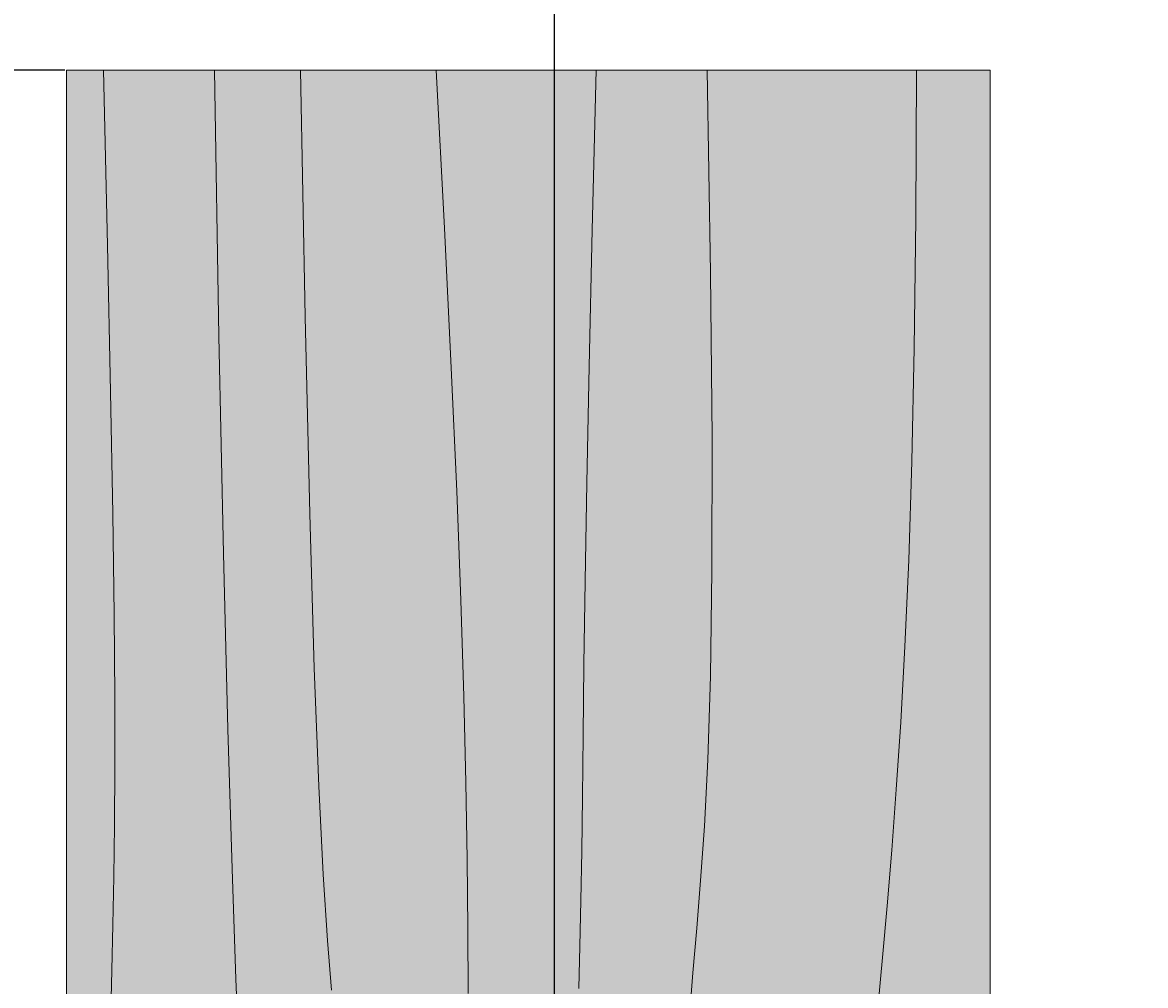
# Model space of a CAD drawing. Units: inches. Extents: x 2549 to 3108, y 1683 to 2362.
# Tile 26 of 30: x 2949 to 2985, y 2049 to 2080. Entities that reach past the tile are written whole.
import ezdxf

# ---------------------------------------------------------------- set-up
doc = ezdxf.new("R2010")
doc.units = ezdxf.units.IN
for name, color, linetype, lineweight in [('A-ANNO-DIMS', 2, 'Continuous', 18), ('A-FURN', 8, 'Continuous', 18), ('A-FURN-PATT', 9, 'Continuous', 13)]:
    doc.layers.add(name, color=color, linetype=linetype, lineweight=lineweight)
doc.layers.add('C-PKNG-VEHI-PATT', color=251, linetype='Continuous', lineweight=13, true_color=0x636466)
doc.layers.add('C-PVMT-PATT', color=9, linetype='Continuous', lineweight=13, true_color=0xc7c8ca)
doc.styles.get("Standard").update_dxf_attribs({"font": 'arial.ttf'})
doc.dimstyles.get("Standard").update_dxf_attribs({"dimtxt": 0.18, "dimasz": 0.18, "dimexe": 0.18, "dimexo": 0.0625, "dimgap": 0.09, "dimtad": 0, "dimtih": 1, "dimtoh": 1, "dimdec": 4, "dimzin": 0, "dimdsep": 46, "dimtxsty": 'Standard', "dimcen": 0.09, "dimadec": 0, "dimazin": 0, "dimtfac": 1, "dimtdec": 4, "dimtofl": 0, "dimtmove": 0, "dimatfit": 3, "dimfxl": 1, "dimtolj": 1, "dimtzin": 0, "dimarcsym": 0})

# ---------------------------------------------------------------- blocks, each defined once
blk = doc.blocks.new('Table - Rectangular Woodgrain 60 x 30 in.')
for p, q in [((0, 0), (0, -30)), ((60, 0), (0, 0)), ((0, -30), (60, -30))]:
    blk.add_line(p, q)
for points in [[(0, -2.4), (4.8155, -2.418), (9.0302, -2.4688), (12.709, -2.5477), (15.9167, -2.65), (18.7181, -2.7711), (21.1781, -2.9063), (23.3616, -3.0508), (25.3333, -3.2), (27.1477, -3.3495), (28.8172, -3.4958), (30.3437, -3.636)], [(0, -9.2), (6.5759, -9.0858), (11.9385, -9.0365), (16.2527, -9.0418), (19.6833, -9.0917), (22.3952, -9.1759), (24.5531, -9.2844), (26.322, -9.4069), (27.8666, -9.5333), (29.3241, -9.6553), (30.7203, -9.7719)], [(0, -12.8), (5.1847, -12.9322), (9.6213, -13.0323), (13.3963, -13.1059), (16.5958, -13.1583), (19.3063, -13.1952), (21.614, -13.2219), (23.6054, -13.2439), (25.3666, -13.2667), (26.9728, -13.2947), (28.4531, -13.3281), (29.8256, -13.3663)], [(0, -18), (5.124, -17.7273), (9.6609, -17.5057), (13.6705, -17.3303), (17.2125, -17.1958), (20.3467, -17.0973), (23.1328, -17.0297), (25.6307, -16.9878), (27.9, -16.9667), (29.9928, -16.9617)], [(0, -22.4), (8.0098, -22.2501), (14.4094, -22.1011), (19.4168, -21.9535), (23.25, -21.8083), (26.1269, -21.6663), (28.2656, -21.5281), (29.884, -21.3947)], [(0, -25.2), (8.6355, -25.0504), (15.7026, -24.9031), (21.4049, -24.7606), (25.9458, -24.625), (29.529, -24.4988), (32.3578, -24.3844)], [(0, -28.8), (5.6867, -28.6681), (10.45, -28.5698), (14.407, -28.5012), (17.675, -28.4584), (20.3711, -28.4374), (22.6125, -28.4344), (24.5164, -28.4455), (26.2, -28.4667), (27.762, -28.4947), (29.2276, -28.5281), (30.6033, -28.5663)]]:
    blk.add_lwpolyline(points)
blk = doc.blocks.new('*D22')
at = {"layer": 'A-ANNO-DIMS', "color": 0, "lineweight": -2, "transparency": 16777216}
for p, q in [((2950.031, 2078.615), (2940.913, 2078.615)), ((2941.093, 2078.435), (2941.093, 2048.798)), ((2941.093, 2018.795), (2941.093, 2048.431)), ((2950.031, 2018.615), (2940.913, 2018.615))]:
    blk.add_line(p, q, dxfattribs=at)
at = {"layer": 'A-ANNO-DIMS', "color": 0, "transparency": 16777216}
for points in [[(2941.063, 2078.435), (2941.123, 2078.435), (2941.093, 2078.615)], [(2941.063, 2018.795), (2941.123, 2018.795), (2941.093, 2018.615)]]:
    blk.add_solid(points, dxfattribs=at)
at = {"layer": 'Defpoints', "color": 0, "transparency": 16777216}
for p in [(2950.093, 2078.615), (2941.093, 2018.615), (2950.093, 2018.615)]:
    blk.add_point(p, dxfattribs=at)
at = {"layer": 'A-ANNO-DIMS', "color": 0, "transparency": 16777216, "insert": (2941.093, 2048.615), "char_height": 0.18, "attachment_point": 5}
blk.add_mtext('\\A1;COFFEE TABLE 60', dxfattribs=at)
blk = doc.blocks.new('*D46')
at = {"layer": 'A-ANNO-DIMS', "color": 0, "lineweight": -2, "transparency": 16777216}
for p, q in [((2812.643, 2140.461), (2812.643, 1683.444)), ((3034.643, 2134.461), (3034.643, 1683.444)), ((2812.823, 1683.624), (2923.353, 1683.624)), ((3034.463, 1683.624), (2923.932, 1683.624))]:
    blk.add_line(p, q, dxfattribs=at)
at = {"layer": 'A-ANNO-DIMS', "color": 0, "transparency": 16777216}
for points in [[(2812.823, 1683.654), (2812.823, 1683.594), (2812.643, 1683.624)], [(3034.463, 1683.654), (3034.463, 1683.594), (3034.643, 1683.624)]]:
    blk.add_solid(points, dxfattribs=at)
at = {"layer": 'Defpoints', "color": 0, "transparency": 16777216}
for p in [(2812.643, 2140.524), (3034.643, 2134.524), (3034.643, 1683.624)]:
    blk.add_point(p, dxfattribs=at)
at = {"layer": 'A-ANNO-DIMS', "color": 0, "transparency": 16777216, "insert": (2923.643, 1683.624), "char_height": 0.18, "attachment_point": 5}
blk.add_mtext('\\A1;222', dxfattribs=at)
blk = doc.blocks.new('*D57')
at = {"layer": 'A-ANNO-DIMS', "color": 0, "lineweight": -2, "transparency": 16777216}
for p, q in [((2965.935, 1936.586), (2965.935, 2362.323)), ((3034.643, 1936.586), (3034.643, 2362.323)), ((2966.115, 2362.143), (2999.912, 2362.143)), ((3034.463, 2362.143), (3000.666, 2362.143))]:
    blk.add_line(p, q, dxfattribs=at)
at = {"layer": 'A-ANNO-DIMS', "color": 0, "transparency": 16777216}
for points in [[(2966.115, 2362.173), (2966.115, 2362.113), (2965.935, 2362.143)], [(3034.463, 2362.173), (3034.463, 2362.113), (3034.643, 2362.143)]]:
    blk.add_solid(points, dxfattribs=at)
at = {"layer": 'Defpoints', "color": 0, "transparency": 16777216}
for p in [(3034.643, 2362.143), (2965.935, 1936.524), (3034.643, 1936.524)]:
    blk.add_point(p, dxfattribs=at)
at = {"layer": 'A-ANNO-DIMS', "color": 0, "transparency": 16777216, "insert": (3000.289, 2362.143), "char_height": 0.18, "attachment_point": 5}
blk.add_mtext('\\A1;68.71', dxfattribs=at)
blk = doc.blocks.new('*D63')
at = {"layer": 'A-ANNO-DIMS', "color": 0, "lineweight": -2, "transparency": 16777216}
for p, q in [((2963.328, 2197.213), (2963.508, 2197.213)), ((2963.508, 2197.213), (2963.508, 2124.675)), ((2963.419, 2003.299), (2963.599, 2003.299)), ((2963.509, 2003.209), (2963.509, 2003.389))]:
    blk.add_line(p, q, dxfattribs=at)
at = {"layer": 'A-ANNO-DIMS', "color": 0, "transparency": 16777216}
blk.add_solid([(2963.538, 2124.675), (2963.478, 2124.675), (2963.508, 2124.495)], dxfattribs=at)
at = {"layer": 'Defpoints', "color": 0, "transparency": 16777216}
for p in [(2963.508, 2124.495), (2963.509, 2003.299)]:
    blk.add_point(p, dxfattribs=at)
at = {"layer": 'A-ANNO-DIMS', "color": 0, "transparency": 16777216, "insert": (2962.654, 2197.213), "char_height": 0.18, "attachment_point": 5}
blk.add_mtext('\\A1;2X R121.2', dxfattribs=at)
blk = doc.blocks.new('*D64')
at = {"layer": 'A-ANNO-DIMS', "color": 0, "lineweight": -2, "transparency": 16777216}
for p, q in [((2919.097, 2052.001), (2919.097, 2052.181)), ((2919.007, 2052.091), (2919.187, 2052.091)), ((3101.897, 2052.091), (3033.527, 2052.091))]:
    blk.add_line(p, q, dxfattribs=at)
at = {"layer": 'A-ANNO-DIMS', "color": 0, "transparency": 16777216}
blk.add_solid([(3033.527, 2052.121), (3033.527, 2052.061), (3033.347, 2052.091)], dxfattribs=at)
at = {"layer": 'Defpoints', "color": 0, "transparency": 16777216}
for p in [(2919.097, 2052.091), (3033.347, 2052.091)]:
    blk.add_point(p, dxfattribs=at)
at = {"layer": 'A-ANNO-DIMS', "color": 0, "transparency": 16777216, "insert": (3102.642, 2052.091), "char_height": 0.18, "attachment_point": 5}
blk.add_mtext('\\A1;2X R114.25', dxfattribs=at)

msp = doc.modelspace()

# ---------------------------------------------------------------- hatches: boundary and pattern name
at = {"layer": 'A-FURN-PATT', "transparency": 33554684}
h = msp.add_hatch(color=256, dxfattribs=at)
h.dxf.hatch_style = 1
h.paths.add_polyline_path([(2951.6587, 2056.0021), (2951.6557, 2058.2435), (2951.6347, 2060.9396), (2951.5919, 2064.2076), (2951.5233, 2068.1646), (2951.425, 2072.9279), (2951.2931, 2078.6146), (2950.0931, 2078.6146), (2950.0931, 2018.6146), (2952.4931, 2018.6146), (2952.0883, 2021.7874), (2951.7676, 2024.5157), (2951.521, 2026.8517), (2951.3389, 2028.848), (2951.2115, 2030.5567), (2951.129, 2032.0303), (2951.0817, 2033.321), (2951.0598, 2034.4813), (2951.0547, 2035.5574), (2951.0634, 2036.5714), (2951.0838, 2037.5393), (2951.1139, 2038.4771), (2951.1519, 2039.4009), (2951.1957, 2040.3266), (2951.2434, 2041.2703), (2951.2931, 2042.248), (2951.343, 2043.2741), (2951.392, 2044.3568), (2951.4396, 2045.5028), (2951.4847, 2046.7188), (2951.5268, 2048.0113), (2951.565, 2049.387), (2951.5984, 2050.8526), (2951.6264, 2052.4146), (2951.6476, 2054.0982)])
h.paths.add_polyline_path([(2955.3325, 2057.2097), (2955.19, 2062.912), (2955.0427, 2069.9791), (2954.8931, 2078.6146), (2951.2931, 2078.6146), (2951.425, 2072.9279), (2951.5233, 2068.1646), (2951.5919, 2064.2076), (2951.6347, 2060.9396), (2951.6557, 2058.2435), (2951.6587, 2056.0021), (2951.6476, 2054.0982), (2951.6264, 2052.4146), (2951.5984, 2050.8526), (2951.565, 2049.387), (2951.5268, 2048.0113), (2951.4847, 2046.7188), (2951.4396, 2045.5028), (2951.392, 2044.3568), (2951.343, 2043.2741), (2951.2931, 2042.248), (2951.2434, 2041.2703), (2951.1957, 2040.3266), (2951.1519, 2039.4009), (2951.1139, 2038.4771), (2951.0838, 2037.5393), (2951.0634, 2036.5714), (2951.0547, 2035.5574), (2951.0598, 2034.4813), (2951.0817, 2033.321), (2951.129, 2032.0303), (2951.2115, 2030.5567), (2951.3389, 2028.848), (2951.521, 2026.8517), (2951.7676, 2024.5157), (2952.0883, 2021.7874), (2952.4931, 2018.6146), (2955.2931, 2018.6146), (2955.302, 2019.3711), (2955.3269, 2020.1382), (2955.3652, 2020.9125), (2955.4139, 2021.6907), (2955.4705, 2022.4692), (2955.5321, 2023.2447), (2955.5961, 2024.0137), (2955.6597, 2024.7729), (2955.7206, 2025.5211), (2955.778, 2026.2663), (2955.8314, 2027.0187), (2955.8806, 2027.7886), (2955.9251, 2028.5862), (2955.9644, 2029.4218), (2955.9984, 2030.3056), (2956.0264, 2031.2479), (2956.048, 2032.2589), (2956.0618, 2033.3479), (2956.0663, 2034.5245), (2956.0598, 2035.7979), (2956.0408, 2037.1776), (2956.0077, 2038.6729), (2955.959, 2040.2933), (2955.8931, 2042.0479), (2955.8091, 2043.9787), (2955.7087, 2046.2568), (2955.5943, 2049.0856), (2955.4681, 2052.6688)])
h.paths.add_polyline_path([(2958.1396, 2059.1978), (2957.992, 2064.2052), (2957.843, 2070.6048), (2957.6931, 2078.6146), (2954.8931, 2078.6146), (2955.0427, 2069.9791), (2955.19, 2062.912), (2955.3325, 2057.2097), (2955.4681, 2052.6688), (2955.5943, 2049.0856), (2955.7087, 2046.2568), (2955.8091, 2043.9787), (2955.8931, 2042.0479), (2955.959, 2040.2933), (2956.0077, 2038.6729), (2956.0408, 2037.1776), (2956.0598, 2035.7979), (2956.0663, 2034.5245), (2956.0618, 2033.3479), (2956.048, 2032.2589), (2956.0264, 2031.2479), (2955.9984, 2030.3056), (2955.9644, 2029.4218), (2955.9251, 2028.5862), (2955.8806, 2027.7886), (2955.8314, 2027.0187), (2955.778, 2026.2663), (2955.7206, 2025.5211), (2955.6597, 2024.7729), (2955.5961, 2024.0137), (2955.5321, 2023.2447), (2955.4705, 2022.4692), (2955.4139, 2021.6907), (2955.3652, 2020.9125), (2955.3269, 2020.1382), (2955.302, 2019.3711), (2955.2931, 2018.6146), (2958.4931, 2018.6146), (2958.3701, 2019.0734), (2958.2967, 2019.5472), (2958.2663, 2020.0323), (2958.2723, 2020.525), (2958.3079, 2021.0217), (2958.3665, 2021.5185), (2958.4416, 2022.0118), (2958.5264, 2022.4979), (2958.6154, 2022.9752), (2958.7072, 2023.45), (2958.8012, 2023.9312), (2958.8973, 2024.4271), (2958.9948, 2024.9465), (2959.0936, 2025.498), (2959.1932, 2026.09), (2959.2931, 2026.7313), (2959.3927, 2027.4274), (2959.49, 2028.1717), (2959.5825, 2028.9546), (2959.6681, 2029.7667), (2959.7443, 2030.5983), (2959.8087, 2031.4399), (2959.8591, 2032.2818), (2959.8931, 2033.1146), (2959.909, 2033.931), (2959.9077, 2034.7334), (2959.8907, 2035.5263), (2959.8598, 2036.3146), (2959.8163, 2037.1029), (2959.7618, 2037.8959), (2959.698, 2038.6982), (2959.6264, 2039.5146), (2959.5483, 2040.3504), (2959.4639, 2041.2131), (2959.3733, 2042.1109), (2959.2764, 2043.0521), (2959.1733, 2044.0449), (2959.0639, 2045.0974), (2958.9483, 2046.2179), (2958.8264, 2047.4146), (2958.6984, 2048.7306), (2958.565, 2050.349), (2958.4268, 2052.4877), (2958.2848, 2055.3646)])
h.paths.add_polyline_path([(2963.0634, 2055.4818), (2962.9958, 2058.2679), (2962.8973, 2061.4021), (2962.7628, 2064.9441), (2962.5874, 2068.9537), (2962.3658, 2073.4906), (2962.0931, 2078.6146), (2957.6931, 2078.6146), (2957.843, 2070.6048), (2957.992, 2064.2052), (2958.1396, 2059.1978), (2958.2848, 2055.3646), (2958.4268, 2052.4877), (2958.565, 2050.349), (2958.6984, 2048.7306), (2958.8264, 2047.4146), (2958.9483, 2046.2179), (2959.0639, 2045.0974), (2959.1733, 2044.0449), (2959.2764, 2043.0521), (2959.3733, 2042.1109), (2959.4639, 2041.2131), (2959.5483, 2040.3504), (2959.6264, 2039.5146), (2959.698, 2038.6982), (2959.7618, 2037.8959), (2959.8163, 2037.1029), (2959.8598, 2036.3146), (2959.8907, 2035.5263), (2959.9077, 2034.7334), (2959.909, 2033.931), (2959.8931, 2033.1146), (2959.8591, 2032.2818), (2959.8087, 2031.4399), (2959.7443, 2030.5983), (2959.6681, 2029.7667), (2959.5825, 2028.9546), (2959.49, 2028.1717), (2959.3927, 2027.4274), (2959.2931, 2026.7313), (2959.1932, 2026.09), (2959.0936, 2025.498), (2958.9948, 2024.9465), (2958.8973, 2024.4271), (2958.8012, 2023.9312), (2958.7072, 2023.45), (2958.6154, 2022.9752), (2958.5264, 2022.4979), (2958.4416, 2022.0118), (2958.3665, 2021.5185), (2958.3079, 2021.0217), (2958.2723, 2020.525), (2958.2663, 2020.0323), (2958.2967, 2019.5472), (2958.3701, 2019.0734), (2958.4931, 2018.6146), (2962.8931, 2018.6146), (2962.8935, 2018.8741), (2962.9256, 2019.0114), (2962.9493, 2019.1068), (2962.9824, 2019.2467), (2963.0264, 2019.448), (2963.082, 2019.7222), (2963.1462, 2020.0607), (2963.2151, 2020.4496), (2963.2847, 2020.875), (2963.3513, 2021.3231), (2963.4108, 2021.78), (2963.4594, 2022.2318), (2963.4931, 2022.6646), (2963.509, 2023.0681), (2963.5077, 2023.4453), (2963.4907, 2023.8031), (2963.4597, 2024.148), (2963.4163, 2024.4866), (2963.3618, 2024.8256), (2963.298, 2025.1716), (2963.2264, 2025.5313), (2963.1488, 2025.9112), (2963.0681, 2026.3175), (2962.9874, 2026.7562), (2962.9098, 2027.2334), (2962.8384, 2027.7551), (2962.7764, 2028.3274), (2962.7269, 2028.9563), (2962.6931, 2029.6479), (2962.6771, 2030.4072), (2962.6775, 2031.2344), (2962.6919, 2032.1288), (2962.7181, 2033.0896), (2962.7536, 2034.116), (2962.7962, 2035.2073), (2962.8435, 2036.3627), (2962.8931, 2037.5813), (2962.9428, 2038.8647), (2962.9905, 2040.224), (2963.0343, 2041.6723), (2963.0723, 2043.2229), (2963.1024, 2044.8892), (2963.1228, 2046.6844), (2963.1314, 2048.6218), (2963.1264, 2050.7146), (2963.1053, 2052.9839)])
h.paths.add_polyline_path([(2967.0608, 2068.9933), (2967.1609, 2073.4299), (2967.2931, 2078.6146), (2962.0931, 2078.6146), (2962.3658, 2073.4906), (2962.5874, 2068.9537), (2962.7628, 2064.9441), (2962.8973, 2061.4021), (2962.9958, 2058.2679), (2963.0634, 2055.4818), (2963.1053, 2052.9839), (2963.1264, 2050.7146), (2963.1314, 2048.6218), (2963.1228, 2046.6844), (2963.1024, 2044.8892), (2963.0723, 2043.2229), (2963.0343, 2041.6723), (2962.9905, 2040.224), (2962.9428, 2038.8647), (2962.8931, 2037.5813), (2962.8435, 2036.3627), (2962.7962, 2035.2073), (2962.7536, 2034.116), (2962.7181, 2033.0896), (2962.6919, 2032.1288), (2962.6775, 2031.2344), (2962.6771, 2030.4072), (2962.6931, 2029.6479), (2962.7269, 2028.9563), (2962.7764, 2028.3274), (2962.8384, 2027.7551), (2962.9098, 2027.2334), (2962.9874, 2026.7562), (2963.0681, 2026.3175), (2963.1488, 2025.9112), (2963.2264, 2025.5313), (2963.298, 2025.1716), (2963.3618, 2024.8256), (2963.4163, 2024.4866), (2963.4597, 2024.148), (2963.4907, 2023.8031), (2963.5077, 2023.4453), (2963.509, 2023.0681), (2963.4931, 2022.6646), (2963.4594, 2022.2318), (2963.4108, 2021.78), (2963.3513, 2021.3231), (2963.2847, 2020.875), (2963.2151, 2020.4496), (2963.1462, 2020.0607), (2963.082, 2019.7222), (2963.0264, 2019.448), (2962.9824, 2019.2467), (2962.9493, 2019.1068), (2962.9256, 2019.0114), (2962.9098, 2018.9438), (2962.9001, 2018.8871), (2962.8952, 2018.8245), (2962.8933, 2018.7393), (2962.8931, 2018.6146), (2966.4931, 2018.6146), (2966.7749, 2019.8457), (2967.0223, 2020.8601), (2967.2384, 2021.6895), (2967.4264, 2022.3657), (2967.5894, 2022.9204), (2967.7306, 2023.3853), (2967.853, 2023.7923), (2967.9598, 2024.173), (2968.0534, 2024.5532), (2968.1337, 2024.9351), (2968.2, 2025.3148), (2968.2514, 2025.6886), (2968.2872, 2026.0526), (2968.3066, 2026.403), (2968.3088, 2026.7361), (2968.2931, 2027.048), (2968.259, 2027.3358), (2968.2077, 2027.6011), (2968.1407, 2027.846), (2968.0598, 2028.073), (2967.9663, 2028.2843), (2967.8618, 2028.4823), (2967.748, 2028.6694), (2967.6264, 2028.8479), (2967.4987, 2029.0209), (2967.367, 2029.1938), (2967.2338, 2029.3729), (2967.1014, 2029.5646), (2966.9721, 2029.775), (2966.8483, 2030.0104), (2966.7323, 2030.2771), (2966.6264, 2030.5813), (2966.5327, 2030.9288), (2966.4514, 2031.324), (2966.3827, 2031.7707), (2966.3264, 2032.273), (2966.2827, 2032.8345), (2966.2514, 2033.4594), (2966.2327, 2034.1515), (2966.2264, 2034.9146), (2966.2324, 2035.7506), (2966.2493, 2036.6521), (2966.2757, 2037.6099), (2966.3098, 2038.6146), (2966.3501, 2039.6568), (2966.3952, 2040.7271), (2966.4434, 2041.8162), (2966.4931, 2042.9146), (2966.543, 2044.0176), (2966.5921, 2045.1386), (2966.6396, 2046.2955), (2966.6848, 2047.5063), (2966.7268, 2048.789), (2966.765, 2050.1615), (2966.7984, 2051.6418), (2966.8264, 2053.248), (2966.8492, 2055.0092), (2966.8712, 2057.0006), (2966.8979, 2059.3083), (2966.9348, 2062.0188), (2966.9872, 2065.2183)])
h.paths.add_polyline_path([(2971.0073, 2072.0387), (2970.8931, 2078.6146), (2967.2931, 2078.6146), (2967.1609, 2073.4299), (2967.0608, 2068.9933), (2966.9872, 2065.2183), (2966.9348, 2062.0188), (2966.8979, 2059.3083), (2966.8712, 2057.0006), (2966.8492, 2055.0092), (2966.8264, 2053.248), (2966.7984, 2051.6418), (2966.765, 2050.1615), (2966.7268, 2048.789), (2966.6848, 2047.5063), (2966.6396, 2046.2955), (2966.5921, 2045.1386), (2966.543, 2044.0176), (2966.4931, 2042.9146), (2966.4434, 2041.8162), (2966.3952, 2040.7271), (2966.3501, 2039.6568), (2966.3098, 2038.6146), (2966.2757, 2037.6099), (2966.2493, 2036.6521), (2966.2324, 2035.7506), (2966.2264, 2034.9146), (2966.2327, 2034.1515), (2966.2514, 2033.4594), (2966.2827, 2032.8345), (2966.3264, 2032.273), (2966.3827, 2031.7707), (2966.4514, 2031.324), (2966.5327, 2030.9288), (2966.6264, 2030.5813), (2966.7323, 2030.2771), (2966.8483, 2030.0104), (2966.9721, 2029.775), (2967.1014, 2029.5646), (2967.2338, 2029.3729), (2967.367, 2029.1938), (2967.4987, 2029.0209), (2967.6264, 2028.8479), (2967.748, 2028.6694), (2967.8618, 2028.4823), (2967.9663, 2028.2843), (2968.0598, 2028.073), (2968.1407, 2027.846), (2968.2077, 2027.6011), (2968.259, 2027.3358), (2968.2931, 2027.048), (2968.3088, 2026.7361), (2968.3066, 2026.403), (2968.2872, 2026.0526), (2968.2514, 2025.6886), (2968.2, 2025.3148), (2968.1337, 2024.9351), (2968.0534, 2024.5532), (2967.9598, 2024.173), (2967.853, 2023.7923), (2967.7306, 2023.3853), (2967.5894, 2022.9204), (2967.4264, 2022.3657), (2967.2384, 2021.6895), (2967.0223, 2020.8601), (2966.7749, 2019.8457), (2966.4931, 2018.6146), (2970.0931, 2018.6146), (2970.5775, 2020.6947), (2971.1181, 2022.524), (2971.6962, 2024.1236), (2972.2931, 2025.5146), (2972.89, 2026.7181), (2973.4681, 2027.7552), (2974.0087, 2028.647), (2974.4931, 2029.4146), (2974.9065, 2030.0774), (2975.2504, 2030.6485), (2975.5302, 2031.139), (2975.7514, 2031.5604), (2975.9195, 2031.924), (2976.04, 2032.2412), (2976.1182, 2032.5231), (2976.1598, 2032.7813), (2976.1697, 2033.0246), (2976.1514, 2033.2532), (2976.1082, 2033.4645), (2976.0431, 2033.6563), (2975.9592, 2033.8262), (2975.8598, 2033.9719), (2975.7478, 2034.091), (2975.6264, 2034.1813), (2975.4975, 2034.241), (2975.3577, 2034.2719), (2975.2022, 2034.2762), (2975.0264, 2034.2563), (2974.8256, 2034.2145), (2974.5952, 2034.1532), (2974.3303, 2034.0746), (2974.0264, 2033.9813), (2973.6814, 2033.8758), (2973.3035, 2033.7625), (2972.9038, 2033.6461), (2972.4931, 2033.5313), (2972.0824, 2033.4227), (2971.6827, 2033.325), (2971.3048, 2033.243), (2970.9598, 2033.1813), (2970.656, 2033.1437), (2970.392, 2033.1302), (2970.1641, 2033.1403), (2969.9681, 2033.173), (2969.8002, 2033.2275), (2969.6566, 2033.3032), (2969.5333, 2033.3991), (2969.4264, 2033.5146), (2969.3328, 2033.6498), (2969.2525, 2033.8084), (2969.1862, 2033.9951), (2969.1348, 2034.2146), (2969.0989, 2034.4716), (2969.0795, 2034.7709), (2969.0773, 2035.117), (2969.0931, 2035.5146), (2969.1271, 2035.9681), (2969.1775, 2036.4802), (2969.2419, 2037.0533), (2969.3181, 2037.6896), (2969.4036, 2038.3916), (2969.4962, 2039.1615), (2969.5935, 2040.0017), (2969.6931, 2040.9146), (2969.7932, 2041.9018), (2969.8941, 2042.962), (2969.9966, 2044.0933), (2970.1014, 2045.2938), (2970.2094, 2046.5614), (2970.3212, 2047.8943), (2970.4378, 2049.2905), (2970.5598, 2050.748), (2970.6862, 2052.2926), (2970.8087, 2054.0615), (2970.9172, 2056.2194), (2971.0014, 2058.9313), (2971.0513, 2062.3619), (2971.0566, 2066.6761)])
h.paths.add_polyline_path([(2977.5454, 2065.9056), (2977.6243, 2069.5844), (2977.6751, 2073.7991), (2977.6931, 2078.6146), (2970.8931, 2078.6146), (2971.0073, 2072.0387), (2971.0566, 2066.6761), (2971.0513, 2062.3619), (2971.0014, 2058.9313), (2970.9172, 2056.2194), (2970.8087, 2054.0615), (2970.6862, 2052.2926), (2970.5598, 2050.748), (2970.4378, 2049.2905), (2970.3212, 2047.8943), (2970.2094, 2046.5614), (2970.1014, 2045.2938), (2969.9966, 2044.0933), (2969.8941, 2042.962), (2969.7932, 2041.9018), (2969.6931, 2040.9146), (2969.5935, 2040.0017), (2969.4962, 2039.1615), (2969.4036, 2038.3916), (2969.3181, 2037.6896), (2969.2419, 2037.0533), (2969.1775, 2036.4802), (2969.1271, 2035.9681), (2969.0931, 2035.5146), (2969.0773, 2035.117), (2969.0795, 2034.7709), (2969.0989, 2034.4716), (2969.1348, 2034.2146), (2969.1862, 2033.9951), (2969.2525, 2033.8084), (2969.3328, 2033.6498), (2969.4264, 2033.5146), (2969.5333, 2033.3991), (2969.6566, 2033.3032), (2969.8002, 2033.2275), (2969.9681, 2033.173), (2970.1641, 2033.1403), (2970.392, 2033.1302), (2970.656, 2033.1437), (2970.9598, 2033.1813), (2971.3048, 2033.243), (2971.6827, 2033.325), (2972.0824, 2033.4227), (2972.4931, 2033.5313), (2972.9038, 2033.6461), (2973.3035, 2033.7625), (2973.6814, 2033.8758), (2974.0264, 2033.9813), (2974.3303, 2034.0746), (2974.5952, 2034.1532), (2974.8256, 2034.2145), (2975.1314, 2034.2781), (2975.4354, 2034.2697), (2975.6264, 2034.1813), (2975.7478, 2034.091), (2975.8598, 2033.9719), (2975.9592, 2033.8262), (2976.0431, 2033.6563), (2976.1082, 2033.4645), (2976.1514, 2033.2532), (2976.1697, 2033.0246), (2976.1598, 2032.7813), (2976.1182, 2032.5231), (2976.04, 2032.2412), (2975.9195, 2031.924), (2975.7514, 2031.5604), (2975.5302, 2031.139), (2975.2504, 2030.6485), (2974.9065, 2030.0774), (2974.4931, 2029.4146), (2974.0087, 2028.647), (2973.4681, 2027.7552), (2972.89, 2026.7181), (2972.2931, 2025.5146), (2971.6962, 2024.1236), (2971.1181, 2022.524), (2970.5775, 2020.6947), (2970.0931, 2018.6146), (2976.8931, 2018.6146), (2977.043, 2020.5019), (2977.192, 2022.3313), (2977.3396, 2024.092), (2977.4848, 2025.773), (2977.6268, 2027.3633), (2977.765, 2028.8521), (2977.8984, 2030.2284), (2978.0264, 2031.4813), (2978.1482, 2032.6032), (2978.2629, 2033.6006), (2978.3698, 2034.483), (2978.4681, 2035.2604), (2978.557, 2035.9425), (2978.6358, 2036.5391), (2978.7036, 2037.0599), (2978.7598, 2037.5146), (2978.8035, 2037.9123), (2978.8348, 2038.2584), (2978.8535, 2038.5576), (2978.8598, 2038.8146), (2978.8535, 2039.0342), (2978.8348, 2039.2209), (2978.8035, 2039.3795), (2978.7598, 2039.5146), (2978.7038, 2039.6302), (2978.6368, 2039.7271), (2978.5605, 2039.8052), (2978.4764, 2039.8646), (2978.3861, 2039.9052), (2978.291, 2039.9271), (2978.1928, 2039.9302), (2978.0931, 2039.9146), (2977.993, 2039.8809), (2977.8921, 2039.8323), (2977.7896, 2039.7728), (2977.6848, 2039.7063), (2977.5003, 2039.5872), (2977.2813, 2039.4666), (2977.0307, 2039.3815), (2976.7627, 2039.3587), (2976.5032, 2039.4189), (2976.3323, 2039.5382), (2976.2264, 2039.648), (2976.1329, 2039.7907), (2976.0535, 2039.9771), (2975.9897, 2040.2198), (2975.9431, 2040.5313), (2975.9152, 2040.924), (2975.9077, 2041.4105), (2975.922, 2042.0032), (2975.9597, 2042.7146), (2976.0217, 2043.5556), (2976.1056, 2044.5297), (2976.2082, 2045.639), (2976.3264, 2046.8855), (2976.4571, 2048.2709), (2976.5973, 2049.7974), (2976.7436, 2051.4669), (2976.8931, 2053.2813), (2977.0423, 2055.253), (2977.1868, 2057.4365), (2977.322, 2059.8965), (2977.4431, 2062.6979)])
h.paths.add_polyline_path([(2980.0931, 2078.6146), (2977.6931, 2078.6146), (2977.6751, 2073.7991), (2977.6243, 2069.5844), (2977.5454, 2065.9056), (2977.4431, 2062.6979), (2977.322, 2059.8965), (2977.1868, 2057.4365), (2977.0423, 2055.253), (2976.8931, 2053.2813), (2976.7436, 2051.4669), (2976.5973, 2049.7974), (2976.4571, 2048.2709), (2976.3264, 2046.8855), (2976.2082, 2045.639), (2976.1056, 2044.5297), (2976.0217, 2043.5556), (2975.9597, 2042.7146), (2975.922, 2042.0032), (2975.9077, 2041.4105), (2975.9152, 2040.924), (2975.9431, 2040.5313), (2975.9897, 2040.2198), (2976.0535, 2039.9771), (2976.1329, 2039.7907), (2976.2264, 2039.648), (2976.3323, 2039.5382), (2976.4483, 2039.4573), (2976.5721, 2039.403), (2976.7014, 2039.373), (2976.8338, 2039.3648), (2976.967, 2039.3761), (2977.0987, 2039.4046), (2977.2264, 2039.448), (2977.3484, 2039.5036), (2977.465, 2039.5678), (2977.5768, 2039.6366), (2977.7721, 2039.7626), (2977.9521, 2039.8671), (2978.144, 2039.9317), (2978.3409, 2039.9255), (2978.5228, 2039.8437), (2978.6765, 2039.6863), (2978.7598, 2039.5146), (2978.8035, 2039.3795), (2978.8348, 2039.2209), (2978.8535, 2039.0342), (2978.8598, 2038.8146), (2978.8535, 2038.5576), (2978.8348, 2038.2584), (2978.8035, 2037.9123), (2978.7598, 2037.5146), (2978.7036, 2037.0599), (2978.6358, 2036.5391), (2978.557, 2035.9425), (2978.4681, 2035.2604), (2978.3698, 2034.483), (2978.2629, 2033.6006), (2978.1482, 2032.6032), (2978.0264, 2031.4813), (2977.8984, 2030.2284), (2977.765, 2028.8521), (2977.6268, 2027.3633), (2977.4848, 2025.773), (2977.3396, 2024.092), (2977.192, 2022.3313), (2977.043, 2020.5019), (2976.8931, 2018.6146), (2980.0931, 2018.6146)])
at = {"layer": 'C-PKNG-VEHI-PATT'}
h = msp.add_hatch(color=256, dxfattribs=at)
h.dxf.hatch_style = 1
edge = h.paths.add_edge_path()
edge.add_ellipse((2935.7258, 1791.964), major_axis=(-50.66, 0), ratio=0.8423039, start_angle=248.16505, end_angle=265.72258)
edge.add_line((2938.911, 1834.5507), (2925.8653, 1834.5507))
edge.add_ellipse((2929.0505, 1791.964), major_axis=(50.66, 0), ratio=0.8423039, start_angle=94.27742, end_angle=111.83495)
edge.add_line((2912.8508, 1832.3947), (2914.2044, 1822.2495))
edge.add_ellipse((2930.6538, 1783.1023), major_axis=(-49.3014, 0), ratio=0.8423039, start_angle=-85.12993, end_angle=-67.20809, ccw=False)
edge.add_line((2927.1247, 1824.5225), (2937.6516, 1824.5225))
edge.add_ellipse((2934.1225, 1783.1023), major_axis=(49.3014, 0), ratio=0.8423039, start_angle=67.20809, end_angle=85.12993, ccw=False)
edge.add_line((2950.5719, 1822.2495), (2951.9255, 1832.3947))
edge = h.paths.add_edge_path()
edge.add_ellipse((2903.4793, 1857.3351), major_axis=(-34.7979, 0), ratio=0.8423039, start_angle=180, end_angle=209.43857)
edge.add_ellipse((2961.297, 1857.3351), major_axis=(34.7979, 0), ratio=0.8423039, start_angle=150.56143, end_angle=180)
edge.add_line((2926.4991, 1857.3351), (2926.4991, 1843.7609))
edge.add_ellipse((2924.1251, 1844.3143), major_axis=(-0.2209, 3.9278), ratio=0.6038336, start_angle=89.00201, end_angle=253.65741, ccw=False)
edge.add_line((2921.7512, 1844.2222), (2921.7512, 1853.3975))
edge.add_line((2921.7512, 1853.3975), (2925.269, 1855.8484))
edge.add_ellipse((2925.4782, 1855.4931), major_axis=(0.4584, 0), ratio=0.8423039, start_angle=90, end_angle=134.48021, ccw=False)
edge.add_line((2925.4782, 1855.8792), (2926.4991, 1855.8792))
edge.add_line((2926.4991, 1855.8792), (2926.4991, 1857.3351))
edge.add_ellipse((2961.297, 1857.3351), major_axis=(34.7979, 0), ratio=0.8423039, start_angle=150.56143, end_angle=180, ccw=False)
edge.add_line((2932.3882, 1873.6501), (2932.3882, 1875.7801))
edge.add_ellipse((2932.3882, 1875.3939), major_axis=(0.4584, 0), ratio=0.8423039, start_angle=90, end_angle=127.93313)
edge.add_line((2932.1366, 1875.7167), (2928.5915, 1873.7564))
edge.add_ellipse((2899.9271, 2002.4692), major_axis=(155.4756, 0), ratio=0.84230387, start_angle=-80.743434, end_angle=-77.445067, ccw=False)
edge.add_ellipse((2949.4402, 1715.2151), major_axis=(-189.1422, 0), ratio=0.84230387, start_angle=-79.790461, end_angle=-77.555373)
edge.add_ellipse((3300.3614, 1852.5642), major_axis=(-386.1662, 0), ratio=0.84230387, start_angle=-2.863715, end_angle=2.198541)
edge.add_ellipse((2929.0505, 1792.5159), major_axis=(-55.6192, 0), ratio=0.8423039, start_angle=-85.91759, end_angle=-72.28005, ccw=False)
edge.add_line((2925.7129, 1839.2798), (2939.0634, 1839.2798))
edge.add_ellipse((2935.7258, 1792.5159), major_axis=(55.6192, 0), ratio=0.8423039, start_angle=72.28005, end_angle=85.91759, ccw=False)
edge.add_ellipse((2564.4149, 1852.5642), major_axis=(-386.1662, 0), ratio=0.84230387, start_angle=177.801459, end_angle=182.863715)
edge.add_ellipse((2915.3361, 1715.2151), major_axis=(189.1422, 0), ratio=0.84230387, start_angle=77.555373, end_angle=79.790461)
edge.add_ellipse((2964.8492, 2002.4692), major_axis=(-155.4756, 0), ratio=0.84230387, start_angle=77.445067, end_angle=80.743434, ccw=False)
edge.add_line((2936.1848, 1873.7564), (2932.6397, 1875.7167))
edge.add_ellipse((2932.3882, 1875.3939), major_axis=(0.4584, 0), ratio=0.8423039, start_angle=52.06687, end_angle=90)
edge.add_line((2932.3882, 1875.7801), (2932.3882, 1873.6501))
edge.add_ellipse((2903.4793, 1857.3351), major_axis=(-34.7979, 0), ratio=0.8423039, start_angle=180, end_angle=209.43857, ccw=False)
edge.add_line((2938.2772, 1857.3351), (2938.2772, 1855.8792))
edge.add_line((2938.2772, 1855.8792), (2939.4059, 1855.8792))
edge.add_ellipse((2939.2981, 1855.4931), major_axis=(-0.4584, 0), ratio=0.8423039, start_angle=225.51979, end_angle=270, ccw=False)
edge.add_line((2939.5903, 1855.7906), (2943.0251, 1853.3975))
edge.add_line((2943.0251, 1853.3975), (2943.0251, 1844.2222))
edge.add_ellipse((2940.6512, 1844.3143), major_axis=(0.2209, 3.9278), ratio=0.6038336, start_angle=106.34259, end_angle=270.99799, ccw=False)
edge.add_line((2938.2772, 1843.7609), (2938.2772, 1857.3351))
edge = h.paths.add_edge_path()
edge.add_ellipse((2932.3882, 1865.1973), major_axis=(91.081, 0), ratio=0.8423039, start_angle=256.401865, end_angle=283.598135, ccw=False)
edge.add_line((2914.2044, 1790.0239), (2914.2044, 1778.3622))
edge.add_ellipse((2932.3882, 1853.5356), major_axis=(91.081, 0), ratio=0.8423039, start_angle=256.401865, end_angle=283.598135)
edge.add_line((2950.5719, 1778.3622), (2950.5719, 1790.0239))
edge = h.paths.add_edge_path()
edge.add_ellipse((2948.7383, 1772.3145), major_axis=(1.8336, 0), ratio=0.8423039, start_angle=0, end_angle=90)
edge.add_line((2948.7383, 1773.859), (2916.038, 1773.859))
edge.add_ellipse((2916.038, 1772.3145), major_axis=(1.8336, 0), ratio=0.8423039, start_angle=90, end_angle=180)
edge.add_line((2914.2044, 1772.3145), (2914.2044, 1760.2558))
edge.add_line((2914.2044, 1760.2558), (2950.5719, 1760.2558))
edge.add_line((2950.5719, 1760.2558), (2950.5719, 1772.3145))
h.paths.add_polyline_path([(2748.8496, 2101.6383), (2798.148, 2101.6383), (2798.148, 2111.4248), (2748.8496, 2111.4248)], flags=9)
h.paths.add_polyline_path([(2685.2081, 2101.489), (2719.3253, 2101.489), (2719.3253, 2111.2819), (2685.2081, 2111.2819)], flags=9)
h.paths.add_polyline_path([(2814.6852, 1907.1328), (2847.8384, 1907.1328), (2847.8384, 1916.9258), (2814.6852, 1916.9258)], flags=9)
h.paths.add_polyline_path([(2814.3906, 1835.5864), (2848.0172, 1835.5864), (2848.0172, 1845.3794), (2814.3906, 1845.3794)], flags=9)
h.paths.add_polyline_path([(2800.5245, 1759.1674), (2853.7435, 1759.1674), (2853.7435, 1768.954), (2800.5245, 1768.954)], flags=9)
h.paths.add_polyline_path([(2972.4611, 1807.3305), (3015.3943, 1807.3305), (3015.3943, 1817.117), (2972.4611, 1817.117)], flags=9)
h.paths.add_polyline_path([(2902.3327, 1888.6731), (2937.9131, 1888.6731), (2937.9131, 1898.4661), (2902.3327, 1898.4661)], flags=9)
h.paths.add_polyline_path([(2712.1779, 1878.9039), (2754.1257, 1878.9039), (2754.1257, 1888.6904), (2712.1779, 1888.6904)], flags=9)
h.paths.add_polyline_path([(2614.0056, 2012.812), (2650.0251, 2012.812), (2650.0251, 2022.4371), (2614.0056, 2022.4371)], flags=9)
h.paths.add_polyline_path([(2713.3129, 2003.1645), (2747.4237, 2003.1645), (2747.4237, 2012.951), (2713.3129, 2012.951)], flags=9)
h.paths.add_polyline_path([(2950.1379, 2001.6934), (2982.2992, 2001.6934), (2982.2992, 2011.48), (2950.1379, 2011.48)], flags=9)
h.paths.add_polyline_path([(2940.864, 2238.5537), (2997.5066, 2238.5537), (2997.5066, 2248.3466), (2940.864, 2248.3466)], flags=9)
h.paths.add_polyline_path([(2821.5457, 2202.8348), (2855.663, 2202.8348), (2855.663, 2212.6278), (2821.5457, 2212.6278)], flags=9)
h.paths.add_polyline_path([(2661.8026, 2238.6249), (2718.4451, 2238.6249), (2718.4451, 2248.4179), (2661.8026, 2248.4179)], flags=9)
at = {"layer": 'C-PVMT-PATT'}
h = msp.add_hatch(color=256, dxfattribs=at)
h.dxf.hatch_style = 1
h.paths.add_polyline_path([(3067.6427, 2305.5237), (2605.6427, 2305.5237), (2605.6427, 2074.5237), (2629.6427, 2074.5237), (2629.6427, 2281.5237), (3043.6427, 2281.5237), (3043.6427, 1885.5237), (3043.6427, 1872.8745), (3031.1672, 1872.8745), (3031.1672, 1862.5731), (2995.8054, 1862.5731), (2995.8054, 1872.8745), (2983.1752, 1872.8745), (2983.1752, 1885.5237), (2881.6427, 1885.5237), (2881.6427, 1795.5237), (2751.0977, 1795.5237), (2751.0977, 1761.5237), (2786.1577, 1761.5237), (2786.1577, 1723.5237), (2881.84, 1723.5237), (2881.84, 1714.5237), (3067.6427, 1714.5237), (3067.6427, 1723.5237)])
edge = h.paths.add_edge_path(flags=16)
edge.add_ellipse((2949.4402, 1710.9683), major_axis=(-194.1014, 0), ratio=0.84230387, start_angle=-77.874034, end_angle=-76.219471, ccw=False)
edge.add_ellipse((2949.4402, 1715.2151), major_axis=(-189.1422, 0), ratio=0.84230387, start_angle=-79.790461, end_angle=-77.555373, ccw=False)
edge.add_ellipse((2899.9271, 2002.4692), major_axis=(155.4756, 0), ratio=0.84230387, start_angle=-80.743434, end_angle=-77.445067)
edge.add_line((2928.5915, 1873.7564), (2932.3882, 1875.8558))
edge.add_line((2932.3882, 1875.8558), (2936.1848, 1873.7564))
edge.add_ellipse((2964.8492, 2002.4692), major_axis=(-155.4756, 0), ratio=0.84230387, start_angle=77.445067, end_angle=80.743434)
edge.add_ellipse((2915.3361, 1715.2151), major_axis=(189.1422, 0), ratio=0.84230387, start_angle=77.555373, end_angle=79.790461, ccw=False)
edge.add_ellipse((2915.3361, 1710.9683), major_axis=(-194.1014, 0), ratio=0.84230387, start_angle=256.219471, end_angle=257.874034, ccw=False)
edge.add_ellipse((2628.2871, 1850.2612), major_axis=(-327.2532, 0), ratio=0.84230387, start_angle=182.17995, end_angle=183.650428, ccw=False)
edge.add_ellipse((2955.5637, 1861.9334), major_axis=(-0.9168, 0), ratio=0.8423039, start_angle=180, end_angle=270, ccw=False)
edge.add_line((2956.4805, 1862.3857), (2956.4805, 1846.4866))
edge.add_ellipse((2955.5637, 1846.939), major_axis=(-0.9168, 0), ratio=0.8423039, start_angle=90, end_angle=180, ccw=False)
edge.add_ellipse((-3607.0606, 1835.832), major_axis=(-6562.6242, 0), ratio=0.84230387, start_angle=179.61613322, end_angle=180.09022909, ccw=False)
edge.add_ellipse((2955.5637, 1791.0926), major_axis=(0.9168, 0), ratio=0.8423039, start_angle=0, end_angle=90, ccw=False)
edge.add_line((2956.4805, 1791.545), (2956.4805, 1775.6459))
edge.add_ellipse((2955.5637, 1776.0982), major_axis=(0.9168, 0), ratio=0.8423039, start_angle=270, end_angle=360, ccw=False)
edge.add_ellipse((-3607.0606, 1835.832), major_axis=(-6562.6242, 0), ratio=0.84230387, start_angle=179.3813568, end_angle=179.47172853, ccw=False)
edge.add_ellipse((2954.5907, 1763.8768), major_axis=(-1.3752, 0), ratio=0.8423039, start_angle=179.37176, end_angle=248.46476, ccw=False)
edge.add_ellipse((-3607.519, 1835.832), major_axis=(-6564.0409, 0), ratio=0.842303863, start_angle=179.35344594, end_angle=179.37176282, ccw=False)
edge.add_ellipse((2952.6829, 1761.8002), major_axis=(3.2503, 0), ratio=0.8423039, start_angle=-90, end_angle=-0.64655, ccw=False)
edge.add_line((2952.6829, 1759.0625), (2912.0934, 1759.0625))
edge.add_ellipse((2912.0934, 1761.8002), major_axis=(3.2503, 0), ratio=0.8423039, start_angle=180.64655, end_angle=270, ccw=False)
edge.add_ellipse((9472.2953, 1835.832), major_axis=(-6564.0409, 0), ratio=0.842303871, start_angle=0.62823722, end_angle=0.6465541, ccw=False)
edge.add_ellipse((2910.1856, 1763.8768), major_axis=(1.3752, 0), ratio=0.8423039, start_angle=111.53524, end_angle=180.62824, ccw=False)
edge.add_ellipse((9471.8369, 1835.832), major_axis=(-6562.6242, 0), ratio=0.84230387, start_angle=0.52827147, end_angle=0.6465541, ccw=False)
edge.add_ellipse((2909.2126, 1776.0982), major_axis=(-0.9168, 0), ratio=0.8423039, start_angle=0, end_angle=90, ccw=False)
edge.add_line((2908.2958, 1775.6459), (2908.2958, 1791.545))
edge.add_ellipse((2909.2126, 1791.0926), major_axis=(-0.9168, 0), ratio=0.8423039, start_angle=-90, end_angle=0, ccw=False)
edge.add_ellipse((9471.8369, 1835.832), major_axis=(-6562.6242, 0), ratio=0.84230387, start_angle=-0.09022909, end_angle=0.38386678, ccw=False)
edge.add_ellipse((2909.2126, 1846.939), major_axis=(-0.9168, 0), ratio=0.8423039, start_angle=0, end_angle=90, ccw=False)
edge.add_line((2908.2958, 1846.4866), (2908.2958, 1862.3857))
edge.add_ellipse((2909.2126, 1861.9334), major_axis=(0.9168, 0), ratio=0.8423039, start_angle=90, end_angle=180, ccw=False)
edge.add_ellipse((3236.4892, 1850.2612), major_axis=(327.2532, 0), ratio=0.84230387, start_angle=176.349572, end_angle=177.82005, ccw=False)
edge = h.paths.add_edge_path(flags=0)
edge.add_ellipse((2903.4793, 1857.3351), major_axis=(-34.7979, 0), ratio=0.8423039, start_angle=180, end_angle=209.43857, ccw=False)
edge.add_line((2938.2772, 1857.3351), (2938.2772, 1855.8792))
edge.add_line((2938.2772, 1855.8792), (2939.4631, 1855.8792))
edge.add_line((2939.4631, 1855.8792), (2943.0251, 1853.3975))
edge.add_line((2943.0251, 1853.3975), (2943.0251, 1844.2222))
edge.add_ellipse((2940.6512, 1844.3143), major_axis=(0.2209, 3.9278), ratio=0.6038336, start_angle=106.34259, end_angle=270.99799, ccw=False)
edge.add_line((2938.2772, 1843.7609), (2938.2772, 1857.3351))
edge.add_ellipse((2903.4793, 1857.3351), major_axis=(-34.7979, 0), ratio=0.8423039, start_angle=180, end_angle=209.43857)
edge.add_ellipse((2961.297, 1857.3351), major_axis=(34.7979, 0), ratio=0.8423039, start_angle=150.56143, end_angle=180)
edge.add_line((2926.4991, 1857.3351), (2926.4991, 1843.7609))
edge.add_ellipse((2924.1251, 1844.3143), major_axis=(-0.2209, 3.9278), ratio=0.6038336, start_angle=89.00201, end_angle=253.65741, ccw=False)
edge.add_line((2921.7512, 1844.2222), (2921.7512, 1853.3975))
edge.add_line((2921.7512, 1853.3975), (2925.3132, 1855.8792))
edge.add_line((2925.3132, 1855.8792), (2926.4991, 1855.8792))
edge.add_line((2926.4991, 1855.8792), (2926.4991, 1857.3351))
edge.add_ellipse((2961.297, 1857.3351), major_axis=(34.7979, 0), ratio=0.8423039, start_angle=150.56143, end_angle=180, ccw=False)
edge = h.paths.add_edge_path(flags=0)
edge.add_ellipse((2929.0505, 1791.964), major_axis=(50.66, 0), ratio=0.8423039, start_angle=94.27742, end_angle=111.83495, ccw=False)
edge.add_line((2925.8653, 1834.5507), (2938.911, 1834.5507))
edge.add_ellipse((2935.7258, 1791.964), major_axis=(-50.66, 0), ratio=0.8423039, start_angle=248.16505, end_angle=265.72258, ccw=False)
edge.add_line((2951.9255, 1832.3947), (2950.5719, 1822.2495))
edge.add_ellipse((2934.1225, 1783.1023), major_axis=(49.3014, 0), ratio=0.8423039, start_angle=67.20809, end_angle=85.12993)
edge.add_line((2937.6516, 1824.5225), (2927.1247, 1824.5225))
edge.add_ellipse((2930.6538, 1783.1023), major_axis=(-49.3014, 0), ratio=0.8423039, start_angle=-85.12993, end_angle=-67.20809)
edge.add_line((2914.2044, 1822.2495), (2912.8508, 1832.3947))
edge = h.paths.add_edge_path(flags=0)
edge.add_line((2910.1338, 1829.4651), (2912.6432, 1821.2711))
edge.add_ellipse((5203.7787, 1816.4367), major_axis=(-2291.1426, 0), ratio=0.84230387, start_angle=-0.1208974, end_angle=0.3640763)
edge.add_line((2912.7012, 1801.8782), (2910.3305, 1792.5698))
edge.add_ellipse((9471.8369, 1835.832), major_axis=(-6561.7074, 0), ratio=0.84230387, start_angle=0.05559431, end_angle=0.37776419, ccw=False)
edge = h.paths.add_edge_path(flags=0)
edge.add_ellipse((-3607.0606, 1835.832), major_axis=(6561.7074, 0), ratio=0.84230387, start_angle=-0.37776419, end_angle=-0.05559431, ccw=False)
edge.add_line((2954.4458, 1792.5698), (2952.0751, 1801.8782))
edge.add_ellipse((660.9976, 1816.4367), major_axis=(2291.1426, 0), ratio=0.84230387, start_angle=-0.3640763, end_angle=0.1208974)
edge.add_line((2952.1331, 1821.2711), (2954.6425, 1829.4651))
edge = h.paths.add_edge_path(flags=0)
edge.add_ellipse((2932.3882, 1865.1973), major_axis=(91.081, 0), ratio=0.8423039, start_angle=256.401865, end_angle=283.598135)
edge.add_line((2950.5719, 1790.0239), (2950.5719, 1778.3622))
edge.add_ellipse((2932.3882, 1853.5356), major_axis=(91.081, 0), ratio=0.8423039, start_angle=256.401865, end_angle=283.598135, ccw=False)
edge.add_line((2914.2044, 1778.3622), (2914.2044, 1790.0239))
edge = h.paths.add_edge_path(flags=0)
edge.add_line((2916.038, 1773.859), (2948.7383, 1773.859))
edge.add_ellipse((2948.7383, 1772.3145), major_axis=(1.8336, 0), ratio=0.8423039, start_angle=0, end_angle=90, ccw=False)
edge.add_line((2950.5719, 1772.3145), (2950.5719, 1760.2558))
edge.add_line((2950.5719, 1760.2558), (2914.2044, 1760.2558))
edge.add_line((2914.2044, 1760.2558), (2914.2044, 1772.3145))
edge.add_ellipse((2916.038, 1772.3145), major_axis=(1.8336, 0), ratio=0.8423039, start_angle=90, end_angle=180, ccw=False)
h.paths.add_polyline_path([(2629.6427, 1978.5237), (2605.6427, 1978.5237), (2605.6427, 1723.5237), (2629.6427, 1723.5237), (2629.6427, 1795.5237)], flags=17)
h.paths.add_polyline_path([(2800.5245, 1759.1674), (2853.7435, 1759.1674), (2853.7435, 1768.954), (2800.5245, 1768.954)], flags=24)
h.paths.add_polyline_path([(2972.4611, 1807.3305), (3015.3943, 1807.3305), (3015.3943, 1817.117), (2972.4611, 1817.117)], flags=24)

# ---------------------------------------------------------------- block references
at = {"layer": 'A-FURN', "rotation": 270}
msp.add_blockref('Table - Rectangular Woodgrain 60 x 30 in.', (2980.0931, 2078.6146), dxfattribs=at)

# ---------------------------------------------------------------- dimensions: what is measured, and where the dimension line sits
at = {"layer": 'A-ANNO-DIMS'}
for base, p1, p2, override, picture, middle in [((3034.6427, 2362.1425), (2965.9351, 1936.5237), (3034.6427, 1936.5237), {"dimdec": 2, "dimlfac": 1, "dimrnd": 0, "dimzin": 0, "dimdsep": 46, "dimlunit": 2}, '*D57', (3000.2889, 2362.1425)), ((3034.6427, 1683.6237), (2812.6427, 2140.5237), (3034.6427, 2134.5237), {"dimdec": 0, "dimlfac": 1, "dimrnd": 0, "dimzin": 0, "dimdsep": 46, "dimlunit": 2}, '*D46', (2923.6427, 1683.6237))]:
    dim = msp.add_linear_dim(base=base, p1=p1, p2=p2, dimstyle='Standard', override=override, dxfattribs=at)
    dim.commit()
    dim.dimension.update_dxf_attribs({"geometry": picture, "text_midpoint": middle})
for center, mpoint, override, picture, middle in [((2963.5085, 2003.2985), (2963.508, 2124.4953), {"dimdec": 1, "dimlfac": 1, "dimrnd": 0, "dimzin": 0, "dimdsep": 46, "dimlunit": 2}, '*D63', (2962.6539, 2197.2134)), ((2919.097, 2052.0905), (3033.347, 2052.091), {"dimdec": 2, "dimlfac": 1, "dimrnd": 0, "dimzin": 0, "dimdsep": 46, "dimlunit": 2}, '*D64', (3101.897, 2052.0913))]:
    dim = msp.add_radius_dim(center=center, mpoint=mpoint, text='2X <>', dimstyle='Standard', override=override, dxfattribs=at)
    dim.commit()
    dim.dimension.update_dxf_attribs({"geometry": picture, "text_midpoint": middle, "dimtype": 164})
dim = msp.add_linear_dim(base=(2941.0931, 2018.6146), p1=(2950.0931, 2078.6146), p2=(2950.0931, 2018.6146), angle=270, text='COFFEE TABLE <>', dimstyle='Standard', override={"dimdec": 0, "dimlfac": 1, "dimrnd": 0, "dimzin": 0, "dimdsep": 46, "dimlunit": 2}, dxfattribs=at)
dim.commit()
dim.dimension.update_dxf_attribs({"geometry": '*D22', "text_midpoint": (2941.0931, 2048.6146)})

doc.saveas('drawing.dxf')
